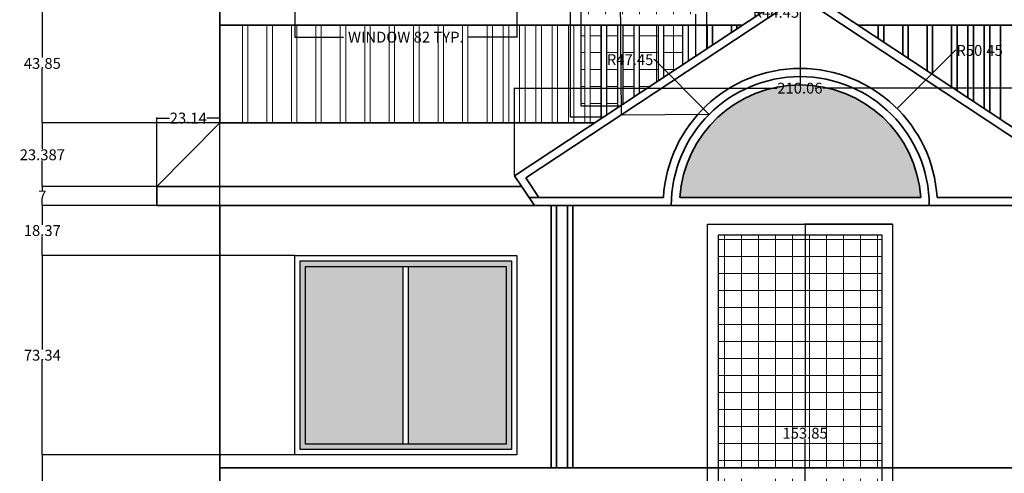
# Model space of a CAD drawing. Units: inches. Extents: x 1366 to 1929, y 372 to 1068.
# Tile 2 of 4: x 1366 to 1728, y 652 to 818. Entities that reach past the tile are written whole.
import ezdxf

# ---------------------------------------------------------------- set-up
doc = ezdxf.new("R2010")
doc.units = ezdxf.units.IN
doc.header["$MEASUREMENT"] = 0
for name, color, linetype, lineweight in [('A-ANNO-DIMS', 2, 'Continuous', 18), ('A-DOOR', 4, 'Continuous', 30), ('A-ELEV', 7, 'Continuous', 35), ('A-ELEV-PATT', 252, 'Continuous', 13), ('A-ELEV-RAIL', 8, 'Continuous', 18), ('A-GLAZ', 4, 'Continuous', 30)]:
    doc.layers.add(name, color=color, linetype=linetype, lineweight=lineweight)
doc.styles.get("Standard").update_dxf_attribs({"font": 'arial.ttf'})
doc.dimstyles.get("Standard").update_dxf_attribs({"dimtxt": 4, "dimasz": 0.18, "dimexe": 0.18, "dimexo": 0.0625, "dimgap": 0.09, "dimtad": 0, "dimtih": 1, "dimtoh": 1, "dimdec": 0, "dimrnd": 6, "dimzin": 0, "dimdsep": 46, "dimlunit": 3, "dimtxsty": 'Standard', "dimcen": 0.09, "dimadec": 0, "dimazin": 0, "dimtfac": 1, "dimtdec": 0, "dimtofl": 0, "dimtmove": 0, "dimatfit": 3, "dimfxl": 1, "dimtolj": 1, "dimtzin": 0, "dimarcsym": 0})

# ---------------------------------------------------------------- blocks, each defined once
blk = doc.blocks.new('WIN-750')
for p, q in [((4, 69.34), (77.81, 69.34)), ((4, 4), (4, 69.34)), ((77.81, 69.34), (77.81, 4)), ((77.81, 4), (4, 4))]:
    blk.add_line(p, q)
for points in [[(0, 73.34), (81.81, 73.34), (81.81, 0), (0, 0)], [(2, 71.34), (79.81, 71.34), (79.81, 2), (2, 2)]]:
    blk.add_lwpolyline(points, close=True)
blk = doc.blocks.new('*D4')
at = {"layer": 'A-ANNO-DIMS', "color": 0, "lineweight": -2, "transparency": 16777216}
for p, q in [((1466.83, 824.16), (1466.83, 811.78)), ((1548.64, 824.16), (1548.64, 811.78)), ((1467.01, 811.96), (1484.79, 811.96)), ((1548.46, 811.96), (1530.67, 811.96))]:
    blk.add_line(p, q, dxfattribs=at)
at = {"layer": 'A-ANNO-DIMS', "color": 0, "lineweight": 30, "transparency": 16777216}
for points in [[(1467.01, 811.99), (1467.01, 811.93), (1466.83, 811.96)], [(1548.46, 811.99), (1548.46, 811.93), (1548.64, 811.96)]]:
    blk.add_solid(points, dxfattribs=at)
at = {"layer": 'Defpoints', "color": 0, "lineweight": 30, "transparency": 16777216}
for p in [(1466.83, 824.23), (1548.64, 824.23), (1548.64, 811.96)]:
    blk.add_point(p, dxfattribs=at)
at = {"layer": 'A-ANNO-DIMS', "color": 0, "transparency": 16777216, "insert": (1507.73, 811.96), "char_height": 4, "attachment_point": 5}
blk.add_mtext('\\A1;WINDOW 82 TYP.', dxfattribs=at)
blk = doc.blocks.new('*D31')
at = {"layer": 'A-ANNO-DIMS', "color": 0, "lineweight": -2, "transparency": 16777216}
for p, q in [((1466.76, 658.28), (1373.77, 658.28)), ((1373.95, 658.1), (1373.95, 638.03)), ((1373.95, 613.69), (1373.95, 633.76)), ((1439.16, 613.51), (1373.77, 613.51))]:
    blk.add_line(p, q, dxfattribs=at)
at = {"layer": 'A-ANNO-DIMS', "color": 0, "lineweight": 30, "transparency": 16777216}
for points in [[(1373.92, 658.1), (1373.98, 658.1), (1373.95, 658.28)], [(1373.92, 613.69), (1373.98, 613.69), (1373.95, 613.51)]]:
    blk.add_solid(points, dxfattribs=at)
at = {"layer": 'Defpoints', "color": 0, "lineweight": 30, "transparency": 16777216}
for p in [(1373.95, 658.28), (1466.83, 658.28), (1439.22, 613.51)]:
    blk.add_point(p, dxfattribs=at)
at = {"layer": 'A-ANNO-DIMS', "color": 0, "transparency": 16777216, "insert": (1373.95, 635.89), "char_height": 4, "attachment_point": 5}
blk.add_mtext('\\A1;44.78', dxfattribs=at)
blk = doc.blocks.new('*D32')
at = {"layer": 'A-ANNO-DIMS', "color": 0, "lineweight": -2, "transparency": 16777216}
for p, q in [((1466.76, 731.62), (1373.77, 731.62)), ((1373.95, 731.44), (1373.95, 697.09)), ((1373.95, 658.46), (1373.95, 692.82)), ((1466.76, 658.28), (1373.77, 658.28))]:
    blk.add_line(p, q, dxfattribs=at)
at = {"layer": 'A-ANNO-DIMS', "color": 0, "lineweight": 30, "transparency": 16777216}
for points in [[(1373.92, 731.44), (1373.98, 731.44), (1373.95, 731.62)], [(1373.92, 658.46), (1373.98, 658.46), (1373.95, 658.28)]]:
    blk.add_solid(points, dxfattribs=at)
at = {"layer": 'Defpoints', "color": 0, "lineweight": 30, "transparency": 16777216}
for p in [(1373.95, 731.62), (1466.83, 731.62), (1466.83, 658.28)]:
    blk.add_point(p, dxfattribs=at)
at = {"layer": 'A-ANNO-DIMS', "color": 0, "transparency": 16777216, "insert": (1373.95, 694.95), "char_height": 4, "attachment_point": 5}
blk.add_mtext('\\A1;73.34', dxfattribs=at)
blk = doc.blocks.new('*D33')
at = {"layer": 'A-ANNO-DIMS', "color": 0, "lineweight": -2, "transparency": 16777216}
for p, q in [((1439.16, 749.99), (1373.77, 749.99)), ((1373.95, 749.81), (1373.95, 742.94)), ((1373.95, 731.8), (1373.95, 738.67)), ((1466.76, 731.62), (1373.77, 731.62))]:
    blk.add_line(p, q, dxfattribs=at)
at = {"layer": 'A-ANNO-DIMS', "color": 0, "lineweight": 30, "transparency": 16777216}
for points in [[(1373.92, 749.81), (1373.98, 749.81), (1373.95, 749.99)], [(1373.92, 731.8), (1373.98, 731.8), (1373.95, 731.62)]]:
    blk.add_solid(points, dxfattribs=at)
at = {"layer": 'Defpoints', "color": 0, "lineweight": 30, "transparency": 16777216}
for p in [(1373.95, 749.99), (1439.22, 749.99), (1466.83, 731.62)]:
    blk.add_point(p, dxfattribs=at)
at = {"layer": 'A-ANNO-DIMS', "color": 0, "transparency": 16777216, "insert": (1373.95, 740.81), "char_height": 4, "attachment_point": 5}
blk.add_mtext('\\A1;18.37', dxfattribs=at)
blk = doc.blocks.new('*D34')
at = {"layer": 'A-ANNO-DIMS', "color": 0, "lineweight": -2, "transparency": 16777216}
for p, q in [((1416.017217, 756.992679), (1373.772656, 756.992679)), ((1373.952656, 756.812679), (1373.952656, 755.582679)), ((1373.952656, 750.172679), (1373.952656, 751.402679)), ((1439.159301, 749.992679), (1373.772656, 749.992679))]:
    blk.add_line(p, q, dxfattribs=at)
at = {"layer": 'A-ANNO-DIMS', "color": 0, "lineweight": 30, "transparency": 16777216}
for points in [[(1373.922656, 756.812679), (1373.982656, 756.812679), (1373.952656, 756.992679)], [(1373.922656, 750.172679), (1373.982656, 750.172679), (1373.952656, 749.992679)]]:
    blk.add_solid(points, dxfattribs=at)
at = {"layer": 'Defpoints', "color": 0, "lineweight": 30, "transparency": 16777216}
for p in [(1373.952656, 756.992679), (1416.079717, 756.992679), (1439.221801, 749.992679)]:
    blk.add_point(p, dxfattribs=at)
at = {"layer": 'A-ANNO-DIMS', "color": 0, "transparency": 16777216, "insert": (1373.952656, 753.492679), "char_height": 4, "attachment_point": 5}
blk.add_mtext('\\A1;7', dxfattribs=at)
blk = doc.blocks.new('*D35')
at = {"layer": 'A-ANNO-DIMS', "color": 0, "lineweight": -2, "transparency": 16777216}
for p, q in [((1439.16, 780.38), (1373.77, 780.38)), ((1373.95, 780.2), (1373.95, 770.82)), ((1373.95, 757.17), (1373.95, 766.55)), ((1416.02, 756.99), (1373.77, 756.99))]:
    blk.add_line(p, q, dxfattribs=at)
at = {"layer": 'A-ANNO-DIMS', "color": 0, "lineweight": 30, "transparency": 16777216}
for points in [[(1373.92, 780.2), (1373.98, 780.2), (1373.95, 780.38)], [(1373.92, 757.17), (1373.98, 757.17), (1373.95, 756.99)]]:
    blk.add_solid(points, dxfattribs=at)
at = {"layer": 'Defpoints', "color": 0, "lineweight": 30, "transparency": 16777216}
for p in [(1373.95, 780.38), (1439.22, 780.38), (1416.08, 756.99)]:
    blk.add_point(p, dxfattribs=at)
at = {"layer": 'A-ANNO-DIMS', "color": 0, "transparency": 16777216, "insert": (1373.95, 768.69), "char_height": 4, "attachment_point": 5}
blk.add_mtext('\\A1;23.387', dxfattribs=at)
blk = doc.blocks.new('*D36')
at = {"layer": 'A-ANNO-DIMS', "color": 0, "lineweight": -2, "transparency": 16777216}
for p, q in [((1466.76, 824.23), (1373.77, 824.23)), ((1373.95, 824.05), (1373.95, 804.44)), ((1373.95, 780.56), (1373.95, 800.17)), ((1439.16, 780.38), (1373.77, 780.38))]:
    blk.add_line(p, q, dxfattribs=at)
at = {"layer": 'A-ANNO-DIMS', "color": 0, "lineweight": 30, "transparency": 16777216}
for points in [[(1373.92, 824.05), (1373.98, 824.05), (1373.95, 824.23)], [(1373.92, 780.56), (1373.98, 780.56), (1373.95, 780.38)]]:
    blk.add_solid(points, dxfattribs=at)
at = {"layer": 'Defpoints', "color": 0, "lineweight": 30, "transparency": 16777216}
for p in [(1373.95, 824.23), (1466.83, 824.23), (1439.22, 780.38)]:
    blk.add_point(p, dxfattribs=at)
at = {"layer": 'A-ANNO-DIMS', "color": 0, "transparency": 16777216, "insert": (1373.95, 802.3), "char_height": 4, "attachment_point": 5}
blk.add_mtext('\\A1;43.85', dxfattribs=at)
blk = doc.blocks.new('*D55')
at = {"layer": 'A-ANNO-DIMS', "color": 0, "lineweight": -2, "transparency": 16777216}
for p, q in [((1416.08, 750.06), (1416.08, 782.37)), ((1416.26, 782.19), (1420.79, 782.19)), ((1439.04, 782.19), (1434.52, 782.19)), ((1439.22, 750.06), (1439.22, 782.37))]:
    blk.add_line(p, q, dxfattribs=at)
at = {"layer": 'A-ANNO-DIMS', "color": 0, "lineweight": 30, "transparency": 16777216}
for points in [[(1416.26, 782.22), (1416.26, 782.16), (1416.08, 782.19)], [(1439.04, 782.22), (1439.04, 782.16), (1439.22, 782.19)]]:
    blk.add_solid(points, dxfattribs=at)
at = {"layer": 'Defpoints', "color": 0, "lineweight": 30, "transparency": 16777216}
for p in [(1439.22, 782.19), (1416.08, 749.99), (1439.22, 749.99)]:
    blk.add_point(p, dxfattribs=at)
at = {"layer": 'A-ANNO-DIMS', "color": 0, "transparency": 16777216, "insert": (1427.65, 782.19), "char_height": 4, "attachment_point": 5}
blk.add_mtext('\\A1;23.14', dxfattribs=at)
blk = doc.blocks.new('*D57')
at = {"layer": 'A-ANNO-DIMS', "color": 0, "lineweight": -2, "transparency": 16777216}
for p, q in [((1618.3, 898.22), (1585.98, 897.94)), ((1586.16, 897.77), (1586.63, 842.74)), ((1587.13, 783.45), (1586.66, 838.48)), ((1619.27, 783.54), (1586.95, 783.27))]:
    blk.add_line(p, q, dxfattribs=at)
at = {"layer": 'A-ANNO-DIMS', "color": 0, "lineweight": 30, "transparency": 16777216}
for points in [[(1586.19, 897.77), (1586.13, 897.77), (1586.16, 897.95)], [(1587.16, 783.45), (1587.1, 783.45), (1587.13, 783.27)]]:
    blk.add_solid(points, dxfattribs=at)
at = {"layer": 'Defpoints', "color": 0, "lineweight": 30, "transparency": 16777216}
for p in [(1586.16, 897.95), (1618.36, 898.22), (1619.33, 783.54)]:
    blk.add_point(p, dxfattribs=at)
at = {"layer": 'A-ANNO-DIMS', "color": 0, "transparency": 16777216, "insert": (1586.65, 840.61), "char_height": 4, "attachment_point": 5}
blk.add_mtext('\\A1;114.68', dxfattribs=at)
blk = doc.blocks.new('*D61')
at = {"layer": 'A-ANNO-DIMS', "color": 0, "lineweight": -2, "transparency": 16777216}
for p, q in [((1686.8, 743.18), (1654.48, 743.18)), ((1654.66, 743), (1654.66, 668.38)), ((1654.66, 589.5), (1654.66, 664.12)), ((1686.8, 589.32), (1654.48, 589.32))]:
    blk.add_line(p, q, dxfattribs=at)
at = {"layer": 'A-ANNO-DIMS', "color": 0, "lineweight": 30, "transparency": 16777216}
for points in [[(1654.63, 743), (1654.69, 743), (1654.66, 743.18)], [(1654.63, 589.5), (1654.69, 589.5), (1654.66, 589.32)]]:
    blk.add_solid(points, dxfattribs=at)
at = {"layer": 'Defpoints', "color": 0, "lineweight": 30, "transparency": 16777216}
for p in [(1654.66, 743.18), (1686.86, 743.18), (1686.86, 589.32)]:
    blk.add_point(p, dxfattribs=at)
at = {"layer": 'A-ANNO-DIMS', "color": 0, "transparency": 16777216, "insert": (1654.66, 666.25), "char_height": 4, "attachment_point": 5}
blk.add_mtext('\\A1;153.85', dxfattribs=at)
blk = doc.blocks.new('*D62')
at = {"layer": 'A-ANNO-DIMS', "color": 0, "lineweight": -2, "transparency": 16777216}
for p, q in [((1547.72, 761.06), (1547.72, 793.37)), ((1547.9, 793.19), (1644.33, 793.19)), ((1757.61, 793.19), (1661.18, 793.19)), ((1757.79, 761.06), (1757.79, 793.37))]:
    blk.add_line(p, q, dxfattribs=at)
at = {"layer": 'A-ANNO-DIMS', "color": 0, "lineweight": 30, "transparency": 16777216}
for points in [[(1547.9, 793.22), (1547.9, 793.16), (1547.72, 793.19)], [(1757.61, 793.22), (1757.61, 793.16), (1757.79, 793.19)]]:
    blk.add_solid(points, dxfattribs=at)
at = {"layer": 'Defpoints', "color": 0, "lineweight": 30, "transparency": 16777216}
for p in [(1757.79, 793.19), (1547.72, 760.99), (1757.79, 760.99)]:
    blk.add_point(p, dxfattribs=at)
at = {"layer": 'A-ANNO-DIMS', "color": 0, "transparency": 16777216, "insert": (1652.75, 793.19), "char_height": 4, "attachment_point": 5}
blk.add_mtext('\\A1;210.06', dxfattribs=at)
blk = doc.blocks.new('*D63')
at = {"layer": 'A-ANNO-DIMS', "color": 0, "lineweight": -2, "transparency": 16777216}
for p, q in [((1709.95, 807.07), (1688.67, 785.79)), ((1710.13, 807.07), (1709.95, 807.07)), ((1652.88, 749.9), (1652.88, 750.08)), ((1652.79, 749.99), (1652.97, 749.99))]:
    blk.add_line(p, q, dxfattribs=at)
at = {"layer": 'A-ANNO-DIMS', "color": 0, "lineweight": 30, "transparency": 16777216}
blk.add_solid([(1688.65, 785.82), (1688.7, 785.77), (1688.55, 785.67)], dxfattribs=at)
at = {"layer": 'Defpoints', "color": 0, "lineweight": 30, "transparency": 16777216}
for p in [(1688.55, 785.67), (1652.88, 749.99)]:
    blk.add_point(p, dxfattribs=at)
at = {"layer": 'A-ANNO-DIMS', "color": 0, "transparency": 16777216, "insert": (1718.9, 807.07), "char_height": 4, "attachment_point": 5}
blk.add_mtext('\\A1;R50.45', dxfattribs=at)
blk = doc.blocks.new('*D64')
at = {"layer": 'A-ANNO-DIMS', "color": 0, "lineweight": -2, "transparency": 16777216}
for p, q in [((1599.03, 803.68), (1599.21, 803.68)), ((1599.21, 803.68), (1619.21, 783.67)), ((1652.88, 749.9), (1652.88, 750.08)), ((1652.79, 749.99), (1652.97, 749.99))]:
    blk.add_line(p, q, dxfattribs=at)
at = {"layer": 'A-ANNO-DIMS', "color": 0, "lineweight": 30, "transparency": 16777216}
blk.add_solid([(1619.23, 783.7), (1619.18, 783.65), (1619.33, 783.55)], dxfattribs=at)
at = {"layer": 'Defpoints', "color": 0, "lineweight": 30, "transparency": 16777216}
for p in [(1619.33, 783.55), (1652.88, 749.99)]:
    blk.add_point(p, dxfattribs=at)
at = {"layer": 'A-ANNO-DIMS', "color": 0, "transparency": 16777216, "insert": (1590.26, 803.68), "char_height": 4, "attachment_point": 5}
blk.add_mtext('\\A1;R47.45', dxfattribs=at)
blk = doc.blocks.new('*D65')
at = {"layer": 'A-ANNO-DIMS', "color": 0, "lineweight": -2, "transparency": 16777216}
for p, q in [((1652.7, 821.11), (1652.88, 821.11)), ((1652.88, 821.11), (1652.88, 794.62)), ((1652.88, 749.9), (1652.88, 750.08)), ((1652.79, 749.99), (1652.97, 749.99))]:
    blk.add_line(p, q, dxfattribs=at)
at = {"layer": 'A-ANNO-DIMS', "color": 0, "lineweight": 30, "transparency": 16777216}
blk.add_solid([(1652.91, 794.62), (1652.85, 794.62), (1652.88, 794.44)], dxfattribs=at)
at = {"layer": 'Defpoints', "color": 0, "lineweight": 30, "transparency": 16777216}
for p in [(1652.88, 794.44), (1652.88, 749.99)]:
    blk.add_point(p, dxfattribs=at)
at = {"layer": 'A-ANNO-DIMS', "color": 0, "transparency": 16777216, "insert": (1643.93, 821.11), "char_height": 4, "attachment_point": 5}
blk.add_mtext('\\A1;R44.45', dxfattribs=at)

msp = doc.modelspace()

# ---------------------------------------------------------------- hatches: boundary and pattern name
at = {"layer": 'A-ELEV-PATT'}
h = msp.add_hatch(color=256, dxfattribs=at)
h.dxf.hatch_style = 1
h.paths.add_polyline_path([(1546.6356, 729.6227), (1468.827, 729.6227), (1468.827, 660.2826), (1546.6356, 660.2826)])
h.paths.add_polyline_path([(1544.6356, 662.2826), (1470.827, 662.2826), (1470.827, 727.6227), (1544.6356, 727.6227)], flags=16)
h.paths.add_polyline_path([(1818.7172, 725.6227), (1748.9085, 725.6227), (1748.9085, 664.2826), (1818.7172, 664.2826)])
h.paths.add_polyline_path([(1750.9085, 723.6227), (1816.7172, 723.6227), (1816.7172, 666.2826), (1750.9085, 666.2826)], flags=16)
h.paths.add_polyline_path([(1546.6356, 895.5665), (1468.827, 895.5665), (1468.827, 826.2264), (1546.6356, 826.2264)])
h.paths.add_polyline_path([(1544.6356, 828.2264), (1470.827, 828.2264), (1470.827, 893.5665), (1544.6356, 893.5665)], flags=16)
h = msp.add_hatch(dxfattribs=at)
h.set_pattern_fill('ANGLE', color=256, scale=25)
h.set_pattern_definition([(0, (0, 0), (0, 6.875), [5, -1.875]), (90, (0, 0), (-6.875, 4e-16), [5, -1.875])])
h.paths.add_polyline_path([(1544.6356, 893.5665), (1508.6356, 893.5665), (1508.6356, 828.2264), (1544.6356, 828.2264)])
h.paths.add_polyline_path([(1506.6356, 727.6227), (1470.827, 727.6227), (1470.827, 662.2826), (1506.6356, 662.2826)])
h.paths.add_polyline_path([(1544.6356, 727.6227), (1508.6356, 727.6227), (1508.6356, 662.2826), (1544.6356, 662.2826)])
h.paths.add_polyline_path([(1608.5338, 752.9927), (1697.2248, 752.9927, 0.93463511)])
h.paths.add_polyline_path([(1682.8585, 567.593), (1622.7881, 567.593), (1622.7881, 535.593), (1682.8585, 535.593)])
h.paths.add_polyline_path([(1782.7172, 723.6227), (1750.9085, 723.6227), (1750.9085, 666.2826), (1782.7172, 666.2826)])
h.paths.add_polyline_path([(1816.7172, 723.6227), (1784.7172, 723.6227), (1784.7172, 666.2826), (1816.7172, 666.2826)])
h.paths.add_polyline_path([(1817.1901, 526.1862), (1739.2847, 526.1862), (1739.2847, 513.1136), (1817.1901, 513.1136)])
h.paths.add_polyline_path([(1565.633, 526.1862), (1487.7276, 526.1862), (1487.7276, 513.1136), (1565.633, 513.1136)])
h = msp.add_hatch(dxfattribs=at)
h.set_pattern_fill('NET', color=256, scale=50)
h.paths.add_polyline_path([(1614.2855, 894.2183), (1572.2896, 894.2183), (1572.2896, 889.0571), (1572.2896, 820.3796), (1614.2855, 820.3796)])
h.paths.add_polyline_path([(1579.6001, 816.3796), (1575.6001, 816.3796), (1575.6001, 786.5447), (1579.6001, 786.5447)])
h.paths.add_polyline_path([(1585.6001, 816.3796), (1581.6001, 816.3796), (1581.6001, 786.5447), (1585.6001, 786.5447)])
h.paths.add_polyline_path([(1591.6001, 816.3796), (1587.6001, 816.3796), (1587.6001, 787.3399), (1591.6001, 789.9826)])
h.paths.add_polyline_path([(1600.6001, 816.3796), (1593.6001, 816.3796), (1593.6001, 791.3039), (1600.6001, 795.9287)])
h.paths.add_polyline_path([(1609.6001, 816.3796), (1602.6001, 816.3796), (1602.6001, 797.2501), (1609.6001, 801.8748)])
h.paths.add_polyline_path([(1573.6001, 816.3796), (1572.2896, 816.3796), (1572.2896, 786.5447), (1573.6001, 786.5447)])
h = msp.add_hatch(dxfattribs=at)
h.set_pattern_fill('NET', color=256, scale=50)
h.paths.add_polyline_path([(1682.8585, 739.1753), (1622.7881, 739.1753), (1622.7881, 653.5057), (1682.8585, 653.5057)])
h.paths.add_polyline_path([(1682.8585, 531.593), (1622.7881, 531.593), (1622.7881, 442.4442), (1682.8585, 442.4442)])
h.paths.add_polyline_path([(1627.6001, 649.5057), (1622.7881, 649.5057), (1622.7881, 589.3234), (1627.6001, 589.3234)])
h.paths.add_polyline_path([(1636.6001, 649.5057), (1629.6001, 649.5057), (1629.6001, 589.3234), (1636.6001, 589.3234)])
h.paths.add_polyline_path([(1645.6001, 649.5057), (1638.6001, 649.5057), (1638.6001, 589.3234), (1645.6001, 589.3234)])
h.paths.add_polyline_path([(1654.6001, 649.5057), (1647.6001, 649.5057), (1647.6001, 589.3234), (1654.6001, 589.3234)])
h.paths.add_polyline_path([(1663.6001, 649.5057), (1656.6001, 649.5057), (1656.6001, 589.3234), (1663.6001, 589.3234)])
h.paths.add_polyline_path([(1672.6001, 649.5057), (1665.6001, 649.5057), (1665.6001, 589.3234), (1672.6001, 589.3234)])
h.paths.add_polyline_path([(1681.6001, 649.5057), (1674.6001, 649.5057), (1674.6001, 589.3234), (1681.6001, 589.3234)])

# ---------------------------------------------------------------- linework, layer by layer
at = {"layer": 'A-DOOR'}
for p, q in [((1618.3601, 898.2183), (1618.3601, 807.6624)), ((1568.2896, 782.5447), (1568.2896, 889.0571)), ((1572.2896, 786.5447), (1572.2896, 889.0571)), ((1614.3601, 820.3796), (1614.3601, 805.0197)), ((1581.6001, 816.3796), (1581.6001, 783.3758)), ((1585.6001, 816.3796), (1585.6001, 786.0185)), ((1587.6001, 816.3796), (1587.6001, 787.3399)), ((1591.6001, 816.3796), (1591.6001, 789.9826)), ((1593.6001, 816.3796), (1593.6001, 791.3039)), ((1600.6001, 816.3796), (1600.6001, 795.9287)), ((1602.6001, 816.3796), (1602.6001, 797.2501)), ((1609.6001, 816.3796), (1609.6001, 801.8748)), ((1611.6001, 816.3796), (1611.6001, 803.1962)), ((1618.6001, 816.3796), (1618.6001, 807.821)), ((1586.3965, 786.5447), (1572.2896, 786.5447)), ((1580.3421, 782.5447), (1568.2896, 782.5447))]:
    msp.add_line(p, q, dxfattribs=at)
for points in [[(1618.7881, 589.3234), (1618.7881, 743.1753), (1686.8585, 743.1753), (1686.8585, 589.3234)], [(1622.7881, 589.3234), (1622.7881, 739.1753), (1682.8585, 739.1753), (1682.8585, 589.3234)]]:
    msp.add_lwpolyline(points, dxfattribs=at)
at = {"layer": 'A-ELEV'}
for p, q in [((1439.2218, 780.3796), (1439.2218, 916.8666)), ((1439.2218, 780.3796), (1439.2218, 916.8666)), ((1652.8793, 830.4686), (1547.7212, 760.9927)), ((1652.8793, 830.4686), (1757.7853, 760.9927)), ((1652.8773, 826.8716), (1551.8874, 760.1496)), ((1652.8773, 826.8716), (1753.6243, 760.1501)), ((1439.2218, 816.3796), (1631.5543, 816.3796)), ((1579.6001, 816.3796), (1579.6001, 782.0544)), ((1620.6001, 816.3796), (1620.6001, 809.1423)), ((1627.6001, 816.3796), (1627.6001, 813.7671)), ((1629.6001, 816.3796), (1629.6001, 815.0884)), ((1674.1531, 816.3796), (1860.9351, 816.3796)), ((1674.6001, 816.3796), (1674.6001, 816.0836)), ((1681.6001, 816.3796), (1681.6001, 811.4477)), ((1683.6001, 816.3796), (1683.6001, 810.1231)), ((1690.6001, 816.3796), (1690.6001, 805.4873)), ((1692.6001, 816.3796), (1692.6001, 804.1627)), ((1699.6001, 816.3796), (1699.6001, 799.5269)), ((1701.6001, 816.3796), (1701.6001, 798.2023)), ((1708.6001, 816.3796), (1708.6001, 793.5664)), ((1710.6001, 816.3796), (1710.6001, 792.2419)), ((1714.6001, 816.3796), (1714.6001, 789.5928)), ((1716.6001, 816.3796), (1716.6001, 788.2683)), ((1720.6001, 816.3796), (1720.6001, 785.6192)), ((1722.6001, 816.3796), (1722.6001, 784.2947)), ((1726.6001, 816.3796), (1726.6001, 781.6456)), ((1439.2218, 780.3796), (1416.0797, 756.9927)), ((1439.2218, 780.3796), (1577.0651, 780.3796)), ((1547.7212, 760.9927), (1555.0482, 749.9927)), ((1550.2181, 762.6558), (1550.2243, 762.6464)), ((1549.3843, 758.4958), (1549.3749, 758.4896)), ((1551.8874, 760.1496), (1556.6545, 752.9927)), ((1416.0797, 756.9927), (1550.3856, 756.9927)), ((1416.0797, 756.9927), (1416.0797, 749.9927)), ((1553.0499, 752.9927), (1602.5217, 752.9927)), ((1608.5338, 752.9927), (1697.2248, 752.9927)), ((1703.2369, 752.9927), (1748.8704, 752.9927)), ((1439.2218, 749.9927), (1416.0797, 749.9927)), ((1439.2218, 613.5057), (1439.2218, 749.9927)), ((1439.2218, 749.9927), (1860.9351, 749.9927)), ((1561.2261, 749.9927), (1561.2261, 653.5057)), ((1563.2261, 749.9927), (1563.2261, 653.5057)), ((1567.2261, 749.9927), (1567.2261, 653.5057)), ((1569.2261, 749.9927), (1569.2261, 653.5057)), ((1439.2218, 653.5057), (1860.9351, 653.5057))]:
    msp.add_line(p, q, dxfattribs=at)
for radius, start, end in [(50.4469, 3.409305, 176.590695), (47.4469, 0, 180), (44.4469, 3.870196, 176.129804)]:
    msp.add_arc((1652.8793, 749.9927), radius, start, end, dxfattribs=at)
at = {"layer": 'A-ELEV-RAIL'}
for p, q in [((1447.6001, 816.3796), (1447.6001, 780.3796)), ((1449.6001, 816.3796), (1449.6001, 780.3796)), ((1456.6001, 816.3796), (1456.6001, 780.3796)), ((1458.6001, 816.3796), (1458.6001, 780.3796)), ((1465.6001, 816.3796), (1465.6001, 780.3796)), ((1467.6001, 816.3796), (1467.6001, 780.3796)), ((1474.6001, 816.3796), (1474.6001, 780.3796)), ((1476.6001, 816.3796), (1476.6001, 780.3796)), ((1483.6001, 816.3796), (1483.6001, 780.3796)), ((1485.6001, 816.3796), (1485.6001, 780.3796)), ((1492.6001, 816.3796), (1492.6001, 780.3796)), ((1494.6001, 816.3796), (1494.6001, 780.3796)), ((1501.6001, 816.3796), (1501.6001, 780.3796)), ((1503.6001, 816.3796), (1503.6001, 780.3796)), ((1510.6001, 816.3796), (1510.6001, 780.3796)), ((1512.6001, 816.3796), (1512.6001, 780.3796)), ((1519.6001, 816.3796), (1519.6001, 780.3796)), ((1521.6001, 816.3796), (1521.6001, 780.3796)), ((1528.6001, 816.3796), (1528.6001, 780.3796)), ((1530.6001, 816.3796), (1530.6001, 780.3796)), ((1537.6001, 816.3796), (1537.6001, 780.3796)), ((1539.6001, 816.3796), (1539.6001, 780.3796)), ((1543.6001, 816.3796), (1543.6001, 780.3796)), ((1545.6001, 816.3796), (1545.6001, 780.3796)), ((1549.6001, 816.3796), (1549.6001, 780.3796)), ((1551.6001, 816.3796), (1551.6001, 780.3796)), ((1555.6001, 816.3796), (1555.6001, 780.3796)), ((1557.6001, 816.3796), (1557.6001, 780.3796)), ((1561.6001, 816.3796), (1561.6001, 780.3796)), ((1563.6001, 816.3796), (1563.6001, 780.3796)), ((1567.6001, 816.3796), (1567.6001, 780.3796)), ((1569.6001, 816.3796), (1569.6001, 780.3796)), ((1573.6001, 816.3796), (1573.6001, 780.3796)), ((1575.6001, 816.3796), (1575.6001, 780.3796))]:
    msp.add_line(p, q, dxfattribs=at)
at = {"layer": 'A-GLAZ'}
for p, q in [((1506.6356, 727.6227), (1506.6356, 662.2826)), ((1508.6356, 727.6227), (1508.6356, 662.2826))]:
    msp.add_line(p, q, dxfattribs=at)

# ---------------------------------------------------------------- block references
msp.add_blockref('WIN-750', (1466.827, 658.283), dxfattribs=at)

# ---------------------------------------------------------------- dimensions: what is measured, and where the dimension line sits
at = {"layer": 'A-ANNO-DIMS'}
for base, p1, p2, angle, override, picture, middle in [((1586.1613, 897.9461), (1619.3293, 783.5427), (1618.3601, 898.2183), 90.484221, {"dimdec": 2, "dimlfac": 1, "dimrnd": 0, "dimzin": 0, "dimdsep": 46, "dimlunit": 2}, '*D57', (1586.6458, 840.6084)), ((1373.9527, 824.2264), (1439.2218, 780.3796), (1466.827, 824.2264), 90, {"dimdec": 2, "dimlfac": 1, "dimrnd": 0, "dimzin": 0, "dimdsep": 46, "dimlunit": 2}, '*D36', (1373.9527, 802.303)), ((1373.9527, 780.3796), (1416.0797, 756.9927), (1439.2218, 780.3796), 90, {"dimdec": 3, "dimlfac": 1, "dimrnd": 0, "dimzin": 0, "dimdsep": 46, "dimlunit": 2}, '*D35', (1373.9527, 768.6861)), ((1373.9527, 756.9927), (1439.2218, 749.9927), (1416.0797, 756.9927), 90, {"dimdec": 0, "dimlfac": 1, "dimrnd": 0, "dimzin": 0, "dimdsep": 46, "dimlunit": 2}, '*D34', (1373.9527, 753.4927)), ((1373.9527, 749.9927), (1466.827, 731.6227), (1439.2218, 749.9927), 90, {"dimdec": 2, "dimlfac": 1, "dimrnd": 0, "dimzin": 0, "dimdsep": 46, "dimlunit": 2}, '*D33', (1373.9527, 740.8077)), ((1654.6585, 743.1753), (1686.8585, 589.3234), (1686.8585, 743.1753), 90, {"dimdec": 2, "dimlfac": 1, "dimrnd": 0, "dimzin": 0, "dimdsep": 46, "dimlunit": 2}, '*D61', (1654.6585, 666.2493)), ((1373.9527, 731.6227), (1466.827, 658.2826), (1466.827, 731.6227), 90, {"dimdec": 2, "dimlfac": 1, "dimrnd": 0, "dimzin": 0, "dimdsep": 46, "dimlunit": 2}, '*D32', (1373.9527, 694.9526)), ((1373.9527, 658.2826), (1439.2218, 613.5057), (1466.827, 658.2826), 90, {"dimdec": 2, "dimlfac": 1, "dimrnd": 0, "dimzin": 0, "dimdsep": 46, "dimlunit": 2}, '*D31', (1373.9527, 635.8941))]:
    dim = msp.add_linear_dim(base=base, p1=p1, p2=p2, angle=angle, dimstyle='Standard', override=override, dxfattribs=at)
    dim.commit()
    dim.dimension.update_dxf_attribs({"geometry": picture, "text_midpoint": middle})
dim = msp.add_linear_dim(base=(1548.6356, 811.9552), p1=(1466.827, 824.2264), p2=(1548.6356, 824.2264), text='WINDOW <> TYP.', dimstyle='Standard', override={"dimdec": 0, "dimlfac": 1, "dimrnd": 0, "dimzin": 0, "dimdsep": 46, "dimlunit": 2}, dxfattribs=at)
dim.commit()
dim.dimension.update_dxf_attribs({"geometry": '*D4', "text_midpoint": (1507.7313, 811.9552)})
for mpoint, picture, middle in [((1652.879, 794.4396), '*D65', (1643.9308, 821.1077)), ((1688.5473, 785.6673), '*D63', (1718.8962, 807.0721)), ((1619.3333, 783.5467), '*D64', (1590.2577, 803.6791))]:
    dim = msp.add_radius_dim(center=(1652.8793, 749.9927), mpoint=mpoint, dimstyle='Standard', override={"dimdec": 2, "dimlfac": 1, "dimrnd": 0, "dimzin": 0, "dimdsep": 46, "dimlunit": 2}, dxfattribs=at)
    dim.commit()
    dim.dimension.update_dxf_attribs({"geometry": picture, "text_midpoint": middle, "dimtype": 164})
for base, p1, p2, picture, middle in [((1757.7853, 793.1927), (1547.7212, 760.9927), (1757.7853, 760.9927), '*D62', (1652.7533, 793.1927)), ((1439.2218, 782.1927), (1416.0797, 749.9927), (1439.2218, 749.9927), '*D55', (1427.6508, 782.1927))]:
    dim = msp.add_linear_dim(base=base, p1=p1, p2=p2, dimstyle='Standard', override={"dimdec": 2, "dimlfac": 1, "dimrnd": 0, "dimzin": 0, "dimdsep": 46, "dimlunit": 2}, dxfattribs=at)
    dim.commit()
    dim.dimension.update_dxf_attribs({"geometry": picture, "text_midpoint": middle})

doc.saveas('drawing.dxf')
